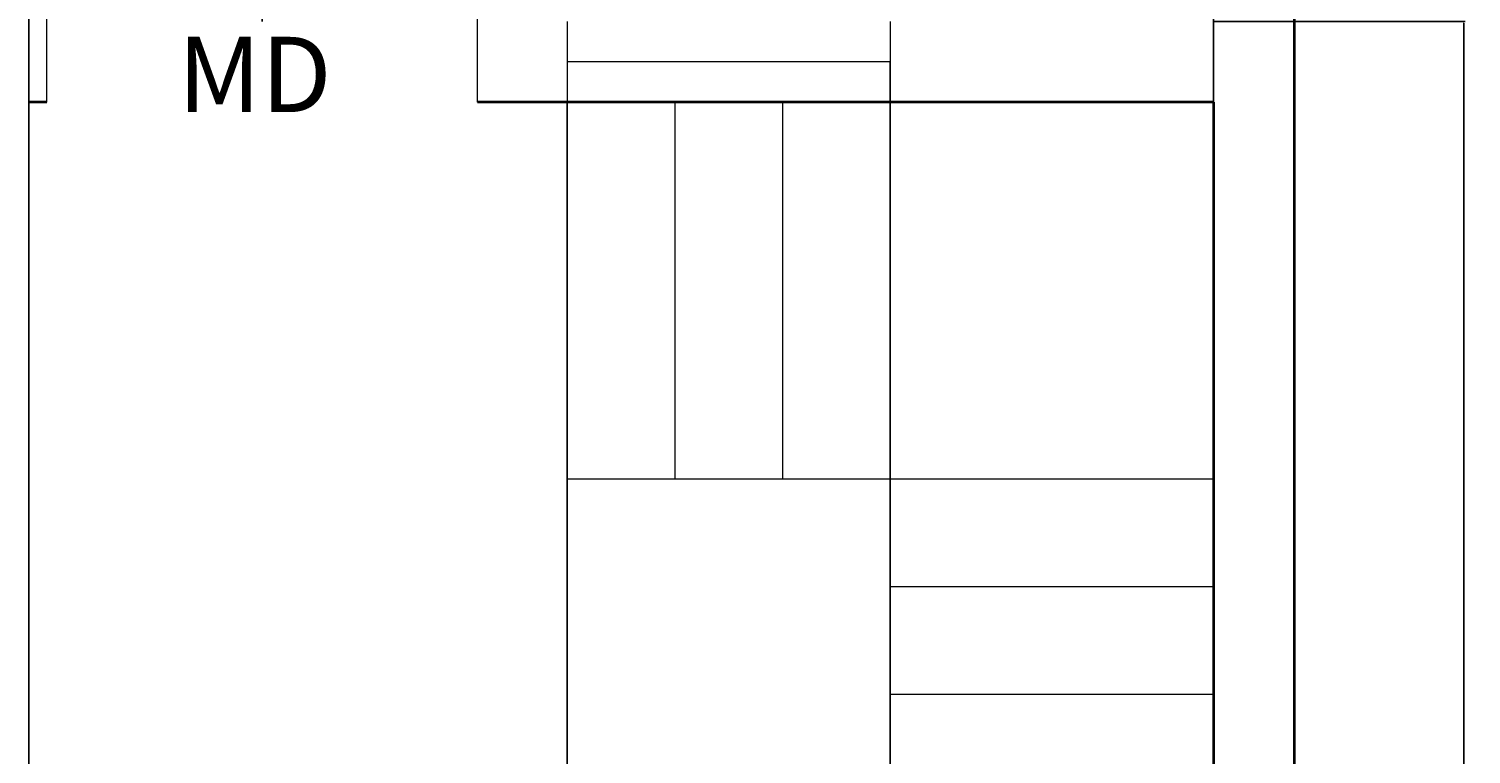
# Model space of a CAD drawing. Units: feet. Extents: x 1654 to 2985, y 1348 to 2230.
# Tile 23 of 53: x 2070 to 2231, y 1670 to 1750. Entities that reach past the tile are written whole.
import ezdxf

# ---------------------------------------------------------------- set-up
doc = ezdxf.new("R2010")
doc.units = ezdxf.units.FT
for name, color, linetype, lineweight in [('A-ANNO-DIMS', 2, 'Continuous', 18), ('A-ANNO-TEXT', 7, 'Continuous', 18), ('A-DOOR', 3, 'Continuous', 18), ('A-FLOR-STRS', 7, 'Continuous', 18), ('A-GLAZ', 4, 'Continuous', 18), ('A-WALL', 7, 'Continuous', 35)]:
    doc.layers.add(name, color=color, linetype=linetype, lineweight=lineweight)
doc.styles.get("Standard").update_dxf_attribs({"font": 'arial.ttf'})
doc.dimstyles.get("Standard").update_dxf_attribs({"dimtxt": 0.18, "dimasz": 0.18, "dimexe": 0.18, "dimexo": 0.0625, "dimgap": 0.09, "dimtad": 0, "dimtih": 1, "dimtoh": 1, "dimdec": 4, "dimzin": 0, "dimdsep": 46, "dimtxsty": 'Standard', "dimcen": 0.09, "dimadec": 0, "dimazin": 0, "dimtfac": 1, "dimtdec": 4, "dimtofl": 0, "dimtmove": 0, "dimatfit": 3, "dimfxl": 1, "dimtolj": 1, "dimtzin": 0, "dimarcsym": 0})

# ---------------------------------------------------------------- blocks, each defined once
blk = doc.blocks.new('DOOR-ENTRY-PAIR')
for p, q in [((0, -9), (0, 24)), ((48, -9), (48, 24))]:
    blk.add_line(p, q)
for centre, start, end in [((0, 0), 0, 90), ((48, 0), 90, 180)]:
    blk.add_arc(centre, 24, start, end)
blk = doc.blocks.new('STAIR-RETURN')
for p, q in [((0, 186), (0, 135)), ((36, 186), (36, 0)), ((0, 177), (0, 135)), ((12, 177), (12, 135)), ((12, 177), (12, 135)), ((24, 177), (24, 135)), ((24, 177), (24, 135)), ((72, 135), (0, 135)), ((72, 123), (36, 123)), ((72, 111), (36, 111)), ((72, 99), (36, 99)), ((72, 87), (36, 87)), ((72, 75), (36, 75)), ((72, 63), (36, 63)), ((72, 51), (36, 51)), ((0, 42), (72, 42)), ((0, 42), (0, 0)), ((12, 42), (12, 0)), ((24, 42), (24, 0))]:
    blk.add_line(p, q)
blk = doc.blocks.new('*D72')
at = {"layer": 'A-ANNO-DIMS', "color": 0, "lineweight": -2, "transparency": 16777216}
for p, q in [((2202.15, 1751.25), (2230.17, 1751.25)), ((2229.99, 1751.07), (2229.99, 1658.44)), ((2229.99, 1565.43), (2229.99, 1658.07)), ((2202.15, 1565.25), (2230.17, 1565.25))]:
    blk.add_line(p, q, dxfattribs=at)
at = {"layer": 'A-ANNO-DIMS', "color": 0, "transparency": 16777216}
for points in [[(2229.96, 1751.07), (2230.02, 1751.07), (2229.99, 1751.25)], [(2229.96, 1565.43), (2230.02, 1565.43), (2229.99, 1565.25)]]:
    blk.add_solid(points, dxfattribs=at)
at = {"layer": 'Defpoints', "color": 0, "transparency": 16777216}
for p in [(2202.09, 1751.25), (2229.99, 1751.25), (2202.09, 1565.25)]:
    blk.add_point(p, dxfattribs=at)
at = {"layer": 'A-ANNO-DIMS', "color": 0, "transparency": 16777216, "insert": (2229.99, 1658.25), "char_height": 0.18, "attachment_point": 5}
blk.add_mtext('\\A1;STAIR 186 TYP.', dxfattribs=at)
blk = doc.blocks.new('*D80')
at = {"layer": 'A-ANNO-DIMS', "color": 0, "lineweight": -2, "transparency": 16777216}
for p, q in [((2070.09, 2039.19), (2070.09, 1534.07)), ((2202.09, 2039.19), (2202.09, 1534.07)), ((2070.27, 1534.25), (2135.81, 1534.25)), ((2201.91, 1534.25), (2136.37, 1534.25))]:
    blk.add_line(p, q, dxfattribs=at)
at = {"layer": 'A-ANNO-DIMS', "color": 0, "transparency": 16777216}
for points in [[(2070.27, 1534.28), (2070.27, 1534.22), (2070.09, 1534.25)], [(2201.91, 1534.28), (2201.91, 1534.22), (2202.09, 1534.25)]]:
    blk.add_solid(points, dxfattribs=at)
at = {"layer": 'Defpoints', "color": 0, "transparency": 16777216}
for p in [(2070.09, 2039.25), (2202.09, 2039.25), (2202.09, 1534.25)]:
    blk.add_point(p, dxfattribs=at)
at = {"layer": 'A-ANNO-DIMS', "color": 0, "transparency": 16777216, "insert": (2136.09, 1534.25), "char_height": 0.18, "attachment_point": 5}
blk.add_mtext('\\A1;132', dxfattribs=at)
blk = doc.blocks.new('*D99')
at = {"layer": 'A-ANNO-DIMS', "color": 0, "lineweight": -2, "transparency": 16777216}
for p, q in [((2166.09, 1746.69), (2166.09, 1534.07)), ((2130.09, 1742.19), (2130.09, 1534.07)), ((2130.27, 1534.25), (2147.87, 1534.25)), ((2165.91, 1534.25), (2148.31, 1534.25))]:
    blk.add_line(p, q, dxfattribs=at)
at = {"layer": 'A-ANNO-DIMS', "color": 0, "transparency": 16777216}
for points in [[(2130.27, 1534.28), (2130.27, 1534.22), (2130.09, 1534.25)], [(2165.91, 1534.28), (2165.91, 1534.22), (2166.09, 1534.25)]]:
    blk.add_solid(points, dxfattribs=at)
at = {"layer": 'Defpoints', "color": 0, "transparency": 16777216}
for p in [(2166.09, 1746.75), (2130.09, 1742.25), (2166.09, 1534.25)]:
    blk.add_point(p, dxfattribs=at)
at = {"layer": 'A-ANNO-DIMS', "color": 0, "transparency": 16777216, "insert": (2148.09, 1534.25), "char_height": 0.18, "attachment_point": 5}
blk.add_mtext('\\A1;36', dxfattribs=at)

msp = doc.modelspace()

# ---------------------------------------------------------------- linework, layer by layer
at = {"layer": 'A-GLAZ'}
msp.add_line((2166.0924, 1746.7549), (2130.0924, 1746.7549), dxfattribs=at)
at = {"layer": 'A-WALL'}
for p, q in [((2211.0924, 2117.2549), (2211.0924, 1742.2549)), ((2211.0924, 1886.2549), (2211.0924, 1565.2549)), ((2072.0924, 1742.2549), (2070.0924, 1742.2549)), ((2202.0924, 1742.2549), (2120.0924, 1742.2549)), ((2202.0924, 1742.2549), (2202.0924, 1565.2549))]:
    msp.add_line(p, q, dxfattribs=at)

# ---------------------------------------------------------------- block references
at = {"layer": 'A-DOOR'}
msp.add_blockref('DOOR-ENTRY-PAIR', (2072.0924, 1751.2549), dxfattribs=at)
at = {"layer": 'A-FLOR-STRS'}
msp.add_blockref('STAIR-RETURN', (2130.092, 1565.255), dxfattribs=at)

# ---------------------------------------------------------------- texts
at = {"layer": 'A-ANNO-TEXT'}
msp.add_text('MD', height=8.38114, dxfattribs=at).set_placement((2086.6849, 1741.1636))

# ---------------------------------------------------------------- dimensions: what is measured, and where the dimension line sits
at = {"layer": 'A-ANNO-DIMS'}
for base, p1, p2, picture, middle in [((2202.0924, 1534.2549), (2070.0924, 2039.2549), (2202.0924, 2039.2549), '*D80', (2136.0924, 1534.2549)), ((2166.0924, 1534.2549), (2130.0924, 1742.2549), (2166.0924, 1746.7549), '*D99', (2148.0924, 1534.2549))]:
    dim = msp.add_linear_dim(base=base, p1=p1, p2=p2, dimstyle='Standard', override={"dimdec": 0, "dimlfac": 1, "dimrnd": 0, "dimzin": 0, "dimdsep": 46, "dimlunit": 2}, dxfattribs=at)
    dim.commit()
    dim.dimension.update_dxf_attribs({"geometry": picture, "text_midpoint": middle})
dim = msp.add_linear_dim(base=(2229.9924, 1751.2549), p1=(2202.0924, 1565.2549), p2=(2202.0924, 1751.2549), angle=90, text='STAIR <> TYP.', dimstyle='Standard', override={"dimdec": 0, "dimlfac": 1, "dimrnd": 0, "dimzin": 0, "dimdsep": 46, "dimlunit": 2}, dxfattribs=at)
dim.commit()
dim.dimension.update_dxf_attribs({"geometry": '*D72', "text_midpoint": (2229.9924, 1658.2549)})

doc.saveas('drawing.dxf')
